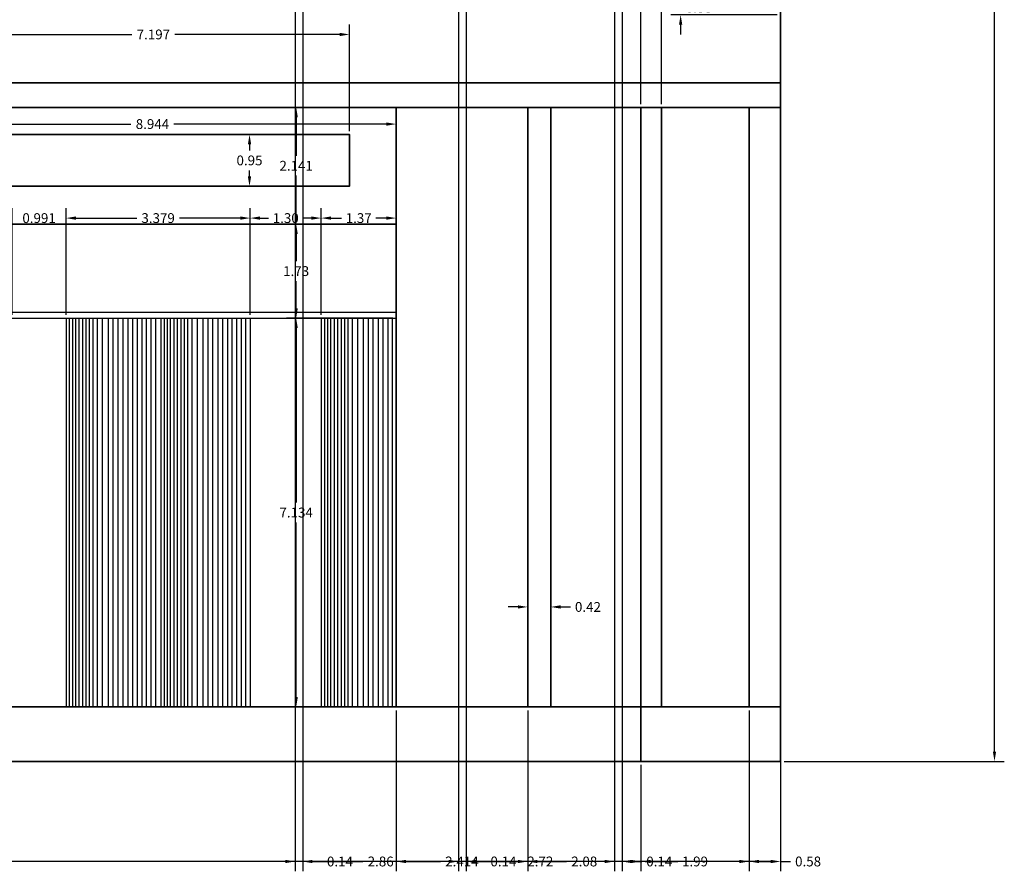
# Model space of a CAD drawing. Units: millimetres. Extents: x 2473 to 2512.3, y 2191.3 to 2230.4.
# Tile 6 of 8: x 2493.7 to 2511.7, y 2191.3 to 2207. Entities that reach past the tile are written whole.
import ezdxf

# ---------------------------------------------------------------- set-up
doc = ezdxf.new("R2010")
doc.units = ezdxf.units.MM
for name, color, linetype, lineweight in [('A-ANNO-DIMS', 2, 'Continuous', 18), ('A-DOOR', 4, 'Continuous', 25), ('A-ELEV', 7, 'Continuous', 35)]:
    doc.layers.add(name, color=color, linetype=linetype, lineweight=lineweight)
doc.styles.get("Standard").update_dxf_attribs({"font": 'arial.ttf'})
doc.dimstyles.get("Standard").update_dxf_attribs({"dimtxt": 0.18, "dimasz": 0.18, "dimexe": 0.18, "dimexo": 0.0625, "dimgap": 0.09, "dimtad": 0, "dimtih": 1, "dimtoh": 1, "dimdec": 4, "dimzin": 0, "dimdsep": 46, "dimtxsty": 'Standard', "dimcen": 0.09, "dimadec": 0, "dimazin": 0, "dimtfac": 1, "dimtdec": 4, "dimtofl": 0, "dimtmove": 0, "dimatfit": 3, "dimfxl": 1, "dimtolj": 1, "dimtzin": 0, "dimarcsym": 0})

# ---------------------------------------------------------------- blocks, each defined once
blk = doc.blocks.new('*D7')
at = {"layer": 'A-ANNO-DIMS', "color": 0, "lineweight": -2, "transparency": 16777216}
for p, q in [((2475.623, 2193.292), (2475.623, 2191.34)), ((2507.623, 2193.292), (2507.623, 2191.34)), ((2475.803, 2191.52), (2491.405, 2191.52)), ((2507.443, 2191.52), (2491.841, 2191.52))]:
    blk.add_line(p, q, dxfattribs=at)
at = {"layer": 'A-ANNO-DIMS', "color": 0, "transparency": 16777216}
for points in [[(2475.803, 2191.55), (2475.803, 2191.49), (2475.623, 2191.52)], [(2507.443, 2191.55), (2507.443, 2191.49), (2507.623, 2191.52)]]:
    blk.add_solid(points, dxfattribs=at)
at = {"layer": 'Defpoints', "color": 0, "transparency": 16777216}
for p in [(2475.623, 2193.355), (2507.623, 2193.355), (2507.623, 2191.52)]:
    blk.add_point(p, dxfattribs=at)
at = {"layer": 'A-ANNO-DIMS', "color": 0, "transparency": 16777216, "insert": (2491.623, 2191.52), "char_height": 0.18, "attachment_point": 5}
blk.add_mtext('\\A1;32', dxfattribs=at)
blk = doc.blocks.new('*D9')
at = {"layer": 'A-ANNO-DIMS', "color": 0, "lineweight": -2, "transparency": 16777216}
for p, q in [((2509.775, 2228.355), (2511.728, 2228.355)), ((2511.548, 2228.175), (2511.548, 2211.037)), ((2511.548, 2193.535), (2511.548, 2210.673)), ((2507.685, 2193.355), (2511.728, 2193.355))]:
    blk.add_line(p, q, dxfattribs=at)
at = {"layer": 'A-ANNO-DIMS', "color": 0, "transparency": 16777216}
for points in [[(2511.518, 2228.175), (2511.578, 2228.175), (2511.548, 2228.355)], [(2511.518, 2193.535), (2511.578, 2193.535), (2511.548, 2193.355)]]:
    blk.add_solid(points, dxfattribs=at)
at = {"layer": 'Defpoints', "color": 0, "transparency": 16777216}
for p in [(2509.713, 2228.355), (2511.548, 2228.355), (2507.623, 2193.355)]:
    blk.add_point(p, dxfattribs=at)
at = {"layer": 'A-ANNO-DIMS', "color": 0, "transparency": 16777216, "insert": (2511.548, 2210.855), "char_height": 0.18, "attachment_point": 5}
blk.add_mtext('\\A1;35', dxfattribs=at)
blk = doc.blocks.new('*D16')
at = {"layer": 'A-ANNO-DIMS', "color": 0, "lineweight": -2, "transparency": 16777216}
for p, q in [((2491.623, 2203.276), (2491.623, 2205.229)), ((2500.567, 2203.276), (2500.567, 2205.229)), ((2491.803, 2205.049), (2495.701, 2205.049)), ((2500.387, 2205.049), (2496.488, 2205.049))]:
    blk.add_line(p, q, dxfattribs=at)
at = {"layer": 'A-ANNO-DIMS', "color": 0, "transparency": 16777216}
for points in [[(2491.803, 2205.079), (2491.803, 2205.019), (2491.623, 2205.049)], [(2500.387, 2205.079), (2500.387, 2205.019), (2500.567, 2205.049)]]:
    blk.add_solid(points, dxfattribs=at)
at = {"layer": 'Defpoints', "color": 0, "transparency": 16777216}
for p in [(2500.567, 2205.049), (2491.623, 2203.214), (2500.567, 2203.214)]:
    blk.add_point(p, dxfattribs=at)
at = {"layer": 'A-ANNO-DIMS', "color": 0, "transparency": 16777216, "insert": (2496.095, 2205.049), "char_height": 0.18, "attachment_point": 5}
blk.add_mtext('\\A1;8.944', dxfattribs=at)
blk = doc.blocks.new('*D26')
at = {"layer": 'A-ANNO-DIMS', "color": 0, "lineweight": -2, "transparency": 16777216}
for p, q in [((2500.567, 2194.292), (2500.567, 2191.34)), ((2502.981, 2194.292), (2502.981, 2191.34)), ((2500.747, 2191.52), (2501.379, 2191.52)), ((2502.801, 2191.52), (2502.169, 2191.52))]:
    blk.add_line(p, q, dxfattribs=at)
at = {"layer": 'A-ANNO-DIMS', "color": 0, "transparency": 16777216}
for points in [[(2500.747, 2191.55), (2500.747, 2191.49), (2500.567, 2191.52)], [(2502.801, 2191.55), (2502.801, 2191.49), (2502.981, 2191.52)]]:
    blk.add_solid(points, dxfattribs=at)
at = {"layer": 'Defpoints', "color": 0, "transparency": 16777216}
for p in [(2500.567, 2194.355), (2502.981, 2194.355), (2502.981, 2191.52)]:
    blk.add_point(p, dxfattribs=at)
at = {"layer": 'A-ANNO-DIMS', "color": 0, "transparency": 16777216, "insert": (2501.774, 2191.52), "char_height": 0.18, "attachment_point": 5}
blk.add_mtext('\\A1;2.414', dxfattribs=at)
blk = doc.blocks.new('*D27')
at = {"layer": 'A-ANNO-DIMS', "color": 0, "lineweight": -2, "transparency": 16777216}
for p, q in [((2502.981, 2194.292), (2502.981, 2191.34)), ((2505.056, 2193.292), (2505.056, 2191.34)), ((2503.161, 2191.52), (2503.693, 2191.52)), ((2504.876, 2191.52), (2504.344, 2191.52))]:
    blk.add_line(p, q, dxfattribs=at)
at = {"layer": 'A-ANNO-DIMS', "color": 0, "transparency": 16777216}
for points in [[(2503.161, 2191.55), (2503.161, 2191.49), (2502.981, 2191.52)], [(2504.876, 2191.55), (2504.876, 2191.49), (2505.056, 2191.52)]]:
    blk.add_solid(points, dxfattribs=at)
at = {"layer": 'Defpoints', "color": 0, "transparency": 16777216}
for p in [(2502.981, 2194.355), (2505.056, 2193.355), (2505.056, 2191.52)]:
    blk.add_point(p, dxfattribs=at)
at = {"layer": 'A-ANNO-DIMS', "color": 0, "transparency": 16777216, "insert": (2504.019, 2191.52), "char_height": 0.18, "attachment_point": 5}
blk.add_mtext('\\A1;2.08', dxfattribs=at)
blk = doc.blocks.new('*D28')
at = {"layer": 'A-ANNO-DIMS', "color": 0, "lineweight": -2, "transparency": 16777216}
for p, q in [((2507.047, 2194.292), (2507.047, 2191.34)), ((2505.056, 2193.292), (2505.056, 2191.34)), ((2505.236, 2191.52), (2505.736, 2191.52)), ((2506.867, 2191.52), (2506.367, 2191.52))]:
    blk.add_line(p, q, dxfattribs=at)
at = {"layer": 'A-ANNO-DIMS', "color": 0, "transparency": 16777216}
for points in [[(2505.236, 2191.55), (2505.236, 2191.49), (2505.056, 2191.52)], [(2506.867, 2191.55), (2506.867, 2191.49), (2507.047, 2191.52)]]:
    blk.add_solid(points, dxfattribs=at)
at = {"layer": 'Defpoints', "color": 0, "transparency": 16777216}
for p in [(2507.047, 2194.355), (2505.056, 2193.355), (2507.047, 2191.52)]:
    blk.add_point(p, dxfattribs=at)
at = {"layer": 'A-ANNO-DIMS', "color": 0, "transparency": 16777216, "insert": (2506.052, 2191.52), "char_height": 0.18, "attachment_point": 5}
blk.add_mtext('\\A1;1.99', dxfattribs=at)
blk = doc.blocks.new('*D29')
at = {"layer": 'A-ANNO-DIMS', "color": 0, "lineweight": -2, "transparency": 16777216}
for p, q in [((2507.047, 2194.292), (2507.047, 2191.34)), ((2507.623, 2194.292), (2507.623, 2191.34)), ((2507.227, 2191.52), (2507.443, 2191.52)), ((2507.623, 2191.52), (2507.803, 2191.52))]:
    blk.add_line(p, q, dxfattribs=at)
at = {"layer": 'A-ANNO-DIMS', "color": 0, "transparency": 16777216}
for points in [[(2507.227, 2191.55), (2507.227, 2191.49), (2507.047, 2191.52)], [(2507.443, 2191.55), (2507.443, 2191.49), (2507.623, 2191.52)]]:
    blk.add_solid(points, dxfattribs=at)
at = {"layer": 'Defpoints', "color": 0, "transparency": 16777216}
for p in [(2507.047, 2194.355), (2507.623, 2194.355), (2507.623, 2191.52)]:
    blk.add_point(p, dxfattribs=at)
at = {"layer": 'A-ANNO-DIMS', "color": 0, "transparency": 16777216, "insert": (2508.127, 2191.52), "char_height": 0.18, "attachment_point": 5}
blk.add_mtext('\\A1;0.58', dxfattribs=at)
blk = doc.blocks.new('*D30')
at = {"layer": 'A-ANNO-DIMS', "color": 0, "lineweight": -2, "transparency": 16777216}
for p, q in [((2502.981, 2194.417), (2502.981, 2196.37)), ((2503.405, 2194.417), (2503.405, 2196.37)), ((2502.801, 2196.19), (2502.621, 2196.19)), ((2503.585, 2196.19), (2503.765, 2196.19))]:
    blk.add_line(p, q, dxfattribs=at)
at = {"layer": 'A-ANNO-DIMS', "color": 0, "transparency": 16777216}
for points in [[(2502.801, 2196.22), (2502.801, 2196.16), (2502.981, 2196.19)], [(2503.585, 2196.22), (2503.585, 2196.16), (2503.405, 2196.19)]]:
    blk.add_solid(points, dxfattribs=at)
at = {"layer": 'Defpoints', "color": 0, "transparency": 16777216}
for p in [(2503.405, 2196.19), (2502.981, 2194.355), (2503.405, 2194.355)]:
    blk.add_point(p, dxfattribs=at)
at = {"layer": 'A-ANNO-DIMS', "color": 0, "transparency": 16777216, "insert": (2504.087, 2196.19), "char_height": 0.18, "attachment_point": 5}
blk.add_mtext('\\A1;0.42', dxfattribs=at)
blk = doc.blocks.new('*D31')
at = {"layer": 'A-ANNO-DIMS', "color": 0, "lineweight": -2, "transparency": 16777216}
for p, q in [((2505.056, 2205.417), (2505.056, 2207.37)), ((2505.438, 2205.417), (2505.438, 2207.37)), ((2504.876, 2207.19), (2504.696, 2207.19)), ((2505.618, 2207.19), (2505.798, 2207.19))]:
    blk.add_line(p, q, dxfattribs=at)
at = {"layer": 'A-ANNO-DIMS', "color": 0, "transparency": 16777216}
for points in [[(2504.876, 2207.22), (2504.876, 2207.16), (2505.056, 2207.19)], [(2505.618, 2207.22), (2505.618, 2207.16), (2505.438, 2207.19)]]:
    blk.add_solid(points, dxfattribs=at)
at = {"layer": 'Defpoints', "color": 0, "transparency": 16777216}
for p in [(2505.438, 2207.19), (2505.056, 2205.355), (2505.438, 2205.355)]:
    blk.add_point(p, dxfattribs=at)
at = {"layer": 'A-ANNO-DIMS', "color": 0, "transparency": 16777216, "insert": (2506.122, 2207.19), "char_height": 0.18, "attachment_point": 5}
blk.add_mtext('\\A1;0.38', dxfattribs=at)
blk = doc.blocks.new('*D33')
at = {"layer": 'A-ANNO-DIMS', "color": 0, "lineweight": -2, "transparency": 16777216}
for p, q in [((2493.518828, 2201.551016), (2493.518828, 2203.503516)), ((2494.509822, 2201.551016), (2494.509822, 2203.503516)), ((2493.338828, 2203.323516), (2493.158828, 2203.323516)), ((2494.689822, 2203.323516), (2494.869822, 2203.323516))]:
    blk.add_line(p, q, dxfattribs=at)
at = {"layer": 'A-ANNO-DIMS', "color": 0, "transparency": 16777216}
for points in [[(2493.338828, 2203.353516), (2493.338828, 2203.293516), (2493.518828, 2203.323516)], [(2494.689822, 2203.353516), (2494.689822, 2203.293516), (2494.509822, 2203.323516)]]:
    blk.add_solid(points, dxfattribs=at)
at = {"layer": 'Defpoints', "color": 0, "transparency": 16777216}
for p in [(2494.509822, 2203.323516), (2493.518828, 2201.488516), (2494.509822, 2201.488516)]:
    blk.add_point(p, dxfattribs=at)
at = {"layer": 'A-ANNO-DIMS', "color": 0, "transparency": 16777216, "insert": (2494.014325, 2203.323516), "char_height": 0.18, "attachment_point": 5}
blk.add_mtext('\\A1;0.991', dxfattribs=at)
blk = doc.blocks.new('*D34')
at = {"layer": 'A-ANNO-DIMS', "color": 0, "lineweight": -2, "transparency": 16777216}
for p, q in [((2494.51, 2201.551), (2494.51, 2203.504)), ((2497.889, 2201.551), (2497.889, 2203.504)), ((2494.69, 2203.324), (2495.806, 2203.324)), ((2497.709, 2203.324), (2496.593, 2203.324))]:
    blk.add_line(p, q, dxfattribs=at)
at = {"layer": 'A-ANNO-DIMS', "color": 0, "transparency": 16777216}
for points in [[(2494.69, 2203.354), (2494.69, 2203.294), (2494.51, 2203.324)], [(2497.709, 2203.354), (2497.709, 2203.294), (2497.889, 2203.324)]]:
    blk.add_solid(points, dxfattribs=at)
at = {"layer": 'Defpoints', "color": 0, "transparency": 16777216}
for p in [(2497.889, 2203.324), (2494.51, 2201.489), (2497.889, 2201.489)]:
    blk.add_point(p, dxfattribs=at)
at = {"layer": 'A-ANNO-DIMS', "color": 0, "transparency": 16777216, "insert": (2496.199, 2203.324), "char_height": 0.18, "attachment_point": 5}
blk.add_mtext('\\A1;3.379', dxfattribs=at)
blk = doc.blocks.new('*D35')
at = {"layer": 'A-ANNO-DIMS', "color": 0, "lineweight": -2, "transparency": 16777216}
for p, q in [((2497.889, 2201.551), (2497.889, 2203.504)), ((2499.192, 2201.551), (2499.192, 2203.504)), ((2498.069, 2203.324), (2498.226, 2203.324)), ((2499.012, 2203.324), (2498.856, 2203.324))]:
    blk.add_line(p, q, dxfattribs=at)
at = {"layer": 'A-ANNO-DIMS', "color": 0, "transparency": 16777216}
for points in [[(2498.069, 2203.354), (2498.069, 2203.294), (2497.889, 2203.324)], [(2499.012, 2203.354), (2499.012, 2203.294), (2499.192, 2203.324)]]:
    blk.add_solid(points, dxfattribs=at)
at = {"layer": 'Defpoints', "color": 0, "transparency": 16777216}
for p in [(2499.192, 2203.324), (2497.889, 2201.489), (2499.192, 2201.489)]:
    blk.add_point(p, dxfattribs=at)
at = {"layer": 'A-ANNO-DIMS', "color": 0, "transparency": 16777216, "insert": (2498.541, 2203.324), "char_height": 0.18, "attachment_point": 5}
blk.add_mtext('\\A1;1.30', dxfattribs=at)
blk = doc.blocks.new('*D36')
at = {"layer": 'A-ANNO-DIMS', "color": 0, "lineweight": -2, "transparency": 16777216}
for p, q in [((2499.192, 2201.551), (2499.192, 2203.504)), ((2500.567, 2201.551), (2500.567, 2203.504)), ((2499.372, 2203.324), (2499.564, 2203.324)), ((2500.387, 2203.324), (2500.195, 2203.324))]:
    blk.add_line(p, q, dxfattribs=at)
at = {"layer": 'A-ANNO-DIMS', "color": 0, "transparency": 16777216}
for points in [[(2499.372, 2203.354), (2499.372, 2203.294), (2499.192, 2203.324)], [(2500.387, 2203.354), (2500.387, 2203.294), (2500.567, 2203.324)]]:
    blk.add_solid(points, dxfattribs=at)
at = {"layer": 'Defpoints', "color": 0, "transparency": 16777216}
for p in [(2500.567, 2203.324), (2499.192, 2201.489), (2500.567, 2201.489)]:
    blk.add_point(p, dxfattribs=at)
at = {"layer": 'A-ANNO-DIMS', "color": 0, "transparency": 16777216, "insert": (2499.88, 2203.324), "char_height": 0.18, "attachment_point": 5}
blk.add_mtext('\\A1;1.37', dxfattribs=at)
blk = doc.blocks.new('*D39')
at = {"layer": 'A-ANNO-DIMS', "color": 0, "lineweight": -2, "transparency": 16777216}
for p, q in [((2500.504, 2201.489), (2498.552, 2201.489)), ((2498.732, 2201.309), (2498.732, 2198.104)), ((2498.732, 2194.535), (2498.732, 2197.74)), ((2500.504, 2194.355), (2498.552, 2194.355))]:
    blk.add_line(p, q, dxfattribs=at)
at = {"layer": 'A-ANNO-DIMS', "color": 0, "transparency": 16777216}
for points in [[(2498.702, 2201.309), (2498.762, 2201.309), (2498.732, 2201.489)], [(2498.702, 2194.535), (2498.762, 2194.535), (2498.732, 2194.355)]]:
    blk.add_solid(points, dxfattribs=at)
at = {"layer": 'Defpoints', "color": 0, "transparency": 16777216}
for p in [(2498.732, 2201.489), (2500.567, 2201.489), (2500.567, 2194.355)]:
    blk.add_point(p, dxfattribs=at)
at = {"layer": 'A-ANNO-DIMS', "color": 0, "transparency": 16777216, "insert": (2498.732, 2197.922), "char_height": 0.18, "attachment_point": 5}
blk.add_mtext('\\A1;7.134', dxfattribs=at)
blk = doc.blocks.new('*D40')
at = {"layer": 'A-ANNO-DIMS', "color": 0, "lineweight": -2, "transparency": 16777216}
for p, q in [((2500.504, 2203.214), (2498.552, 2203.214)), ((2498.732, 2203.034), (2498.732, 2202.533)), ((2498.732, 2201.669), (2498.732, 2202.169)), ((2500.504, 2201.489), (2498.552, 2201.489))]:
    blk.add_line(p, q, dxfattribs=at)
at = {"layer": 'A-ANNO-DIMS', "color": 0, "transparency": 16777216}
for points in [[(2498.702, 2203.034), (2498.762, 2203.034), (2498.732, 2203.214)], [(2498.702, 2201.669), (2498.762, 2201.669), (2498.732, 2201.489)]]:
    blk.add_solid(points, dxfattribs=at)
at = {"layer": 'Defpoints', "color": 0, "transparency": 16777216}
for p in [(2498.732, 2203.214), (2500.567, 2203.214), (2500.567, 2201.489)]:
    blk.add_point(p, dxfattribs=at)
at = {"layer": 'A-ANNO-DIMS', "color": 0, "transparency": 16777216, "insert": (2498.732, 2202.351), "char_height": 0.18, "attachment_point": 5}
blk.add_mtext('\\A1;1.73', dxfattribs=at)
blk = doc.blocks.new('*D41')
at = {"layer": 'A-ANNO-DIMS', "color": 0, "lineweight": -2, "transparency": 16777216}
for p, q in [((2500.504, 2205.355), (2498.552, 2205.355)), ((2498.732, 2205.175), (2498.732, 2204.465)), ((2498.732, 2203.394), (2498.732, 2204.104)), ((2500.504, 2203.214), (2498.552, 2203.214))]:
    blk.add_line(p, q, dxfattribs=at)
at = {"layer": 'A-ANNO-DIMS', "color": 0, "transparency": 16777216}
for points in [[(2498.702, 2205.175), (2498.762, 2205.175), (2498.732, 2205.355)], [(2498.702, 2203.394), (2498.762, 2203.394), (2498.732, 2203.214)]]:
    blk.add_solid(points, dxfattribs=at)
at = {"layer": 'Defpoints', "color": 0, "transparency": 16777216}
for p in [(2498.732, 2205.355), (2500.567, 2205.355), (2500.567, 2203.214)]:
    blk.add_point(p, dxfattribs=at)
at = {"layer": 'A-ANNO-DIMS', "color": 0, "transparency": 16777216, "insert": (2498.732, 2204.284), "char_height": 0.18, "attachment_point": 5}
blk.add_mtext('\\A1;2.141', dxfattribs=at)
blk = doc.blocks.new('*D42')
at = {"layer": 'A-ANNO-DIMS', "color": 0, "lineweight": -2, "transparency": 16777216}
for p, q in [((2499.648, 2204.858), (2497.696, 2204.858)), ((2497.876, 2204.678), (2497.876, 2204.564)), ((2497.876, 2204.087), (2497.876, 2204.2)), ((2499.648, 2203.907), (2497.696, 2203.907))]:
    blk.add_line(p, q, dxfattribs=at)
at = {"layer": 'A-ANNO-DIMS', "color": 0, "transparency": 16777216}
for points in [[(2497.846, 2204.678), (2497.906, 2204.678), (2497.876, 2204.858)], [(2497.846, 2204.087), (2497.906, 2204.087), (2497.876, 2203.907)]]:
    blk.add_solid(points, dxfattribs=at)
at = {"layer": 'Defpoints', "color": 0, "transparency": 16777216}
for p in [(2497.876, 2204.858), (2499.711, 2204.858), (2499.711, 2203.907)]:
    blk.add_point(p, dxfattribs=at)
at = {"layer": 'A-ANNO-DIMS', "color": 0, "transparency": 16777216, "insert": (2497.876, 2204.382), "char_height": 0.18, "attachment_point": 5}
blk.add_mtext('\\A1;0.95', dxfattribs=at)
blk = doc.blocks.new('*D44')
at = {"layer": 'A-ANNO-DIMS', "color": 0, "lineweight": -2, "transparency": 16777216}
for p, q in [((2492.513, 2204.92), (2492.513, 2206.873)), ((2499.711, 2204.92), (2499.711, 2206.873)), ((2492.693, 2206.693), (2495.719, 2206.693)), ((2499.531, 2206.693), (2496.505, 2206.693))]:
    blk.add_line(p, q, dxfattribs=at)
at = {"layer": 'A-ANNO-DIMS', "color": 0, "transparency": 16777216}
for points in [[(2492.693, 2206.723), (2492.693, 2206.663), (2492.513, 2206.693)], [(2499.531, 2206.723), (2499.531, 2206.663), (2499.711, 2206.693)]]:
    blk.add_solid(points, dxfattribs=at)
at = {"layer": 'Defpoints', "color": 0, "transparency": 16777216}
for p in [(2499.711, 2206.693), (2492.513, 2204.858), (2499.711, 2204.858)]:
    blk.add_point(p, dxfattribs=at)
at = {"layer": 'A-ANNO-DIMS', "color": 0, "transparency": 16777216, "insert": (2496.112, 2206.693), "char_height": 0.18, "attachment_point": 5}
blk.add_mtext('\\A1;7.197', dxfattribs=at)
blk = doc.blocks.new('*D61')
at = {"layer": 'A-ANNO-DIMS', "color": 0, "lineweight": -2, "transparency": 16777216}
for p, q in [((2505.788, 2207.687), (2505.788, 2207.867)), ((2507.56, 2207.507), (2505.608, 2207.507)), ((2507.56, 2207.055), (2505.608, 2207.055)), ((2505.788, 2206.875), (2505.788, 2206.695))]:
    blk.add_line(p, q, dxfattribs=at)
at = {"layer": 'A-ANNO-DIMS', "color": 0, "transparency": 16777216}
for points in [[(2505.758, 2207.687), (2505.818, 2207.687), (2505.788, 2207.507)], [(2505.758, 2206.875), (2505.818, 2206.875), (2505.788, 2207.055)]]:
    blk.add_solid(points, dxfattribs=at)
at = {"layer": 'Defpoints', "color": 0, "transparency": 16777216}
for p in [(2505.788, 2207.507), (2507.623, 2207.507), (2507.623, 2207.055)]:
    blk.add_point(p, dxfattribs=at)
at = {"layer": 'A-ANNO-DIMS', "color": 0, "transparency": 16777216, "insert": (2505.788, 2207.281), "char_height": 0.18, "attachment_point": 5}
blk.add_mtext('\\A1;0.452', dxfattribs=at)
blk = doc.blocks.new('*D115')
at = {"layer": 'A-ANNO-DIMS', "color": 0, "lineweight": -2, "transparency": 16777216}
for p, q in [((2498.713, 2222.992), (2498.713, 2191.34)), ((2498.852, 2222.992), (2498.852, 2191.34)), ((2498.533, 2191.52), (2498.353, 2191.52)), ((2499.032, 2191.52), (2499.212, 2191.52))]:
    blk.add_line(p, q, dxfattribs=at)
at = {"layer": 'A-ANNO-DIMS', "color": 0, "transparency": 16777216}
for points in [[(2498.533, 2191.55), (2498.533, 2191.49), (2498.713, 2191.52)], [(2499.032, 2191.55), (2499.032, 2191.49), (2498.852, 2191.52)]]:
    blk.add_solid(points, dxfattribs=at)
at = {"layer": 'Defpoints', "color": 0, "transparency": 16777216}
for p in [(2498.713, 2223.055), (2498.852, 2223.055), (2498.852, 2191.52)]:
    blk.add_point(p, dxfattribs=at)
at = {"layer": 'A-ANNO-DIMS', "color": 0, "transparency": 16777216, "insert": (2499.536, 2191.52), "char_height": 0.18, "attachment_point": 5}
blk.add_mtext('\\A1;0.14', dxfattribs=at)
blk = doc.blocks.new('*D116')
at = {"layer": 'A-ANNO-DIMS', "color": 0, "lineweight": -2, "transparency": 16777216}
for p, q in [((2498.852, 2222.992), (2498.852, 2191.34)), ((2501.713, 2222.992), (2501.713, 2191.34)), ((2499.032, 2191.52), (2499.957, 2191.52)), ((2501.533, 2191.52), (2500.608, 2191.52))]:
    blk.add_line(p, q, dxfattribs=at)
at = {"layer": 'A-ANNO-DIMS', "color": 0, "transparency": 16777216}
for points in [[(2499.032, 2191.55), (2499.032, 2191.49), (2498.852, 2191.52)], [(2501.533, 2191.55), (2501.533, 2191.49), (2501.713, 2191.52)]]:
    blk.add_solid(points, dxfattribs=at)
at = {"layer": 'Defpoints', "color": 0, "transparency": 16777216}
for p in [(2498.852, 2223.055), (2501.713, 2223.055), (2501.713, 2191.52)]:
    blk.add_point(p, dxfattribs=at)
at = {"layer": 'A-ANNO-DIMS', "color": 0, "transparency": 16777216, "insert": (2500.283, 2191.52), "char_height": 0.18, "attachment_point": 5}
blk.add_mtext('\\A1;2.86', dxfattribs=at)
blk = doc.blocks.new('*D117')
at = {"layer": 'A-ANNO-DIMS', "color": 0, "lineweight": -2, "transparency": 16777216}
for p, q in [((2501.713, 2222.992), (2501.713, 2191.34)), ((2501.853, 2222.992), (2501.853, 2191.34)), ((2501.533, 2191.52), (2501.353, 2191.52)), ((2502.033, 2191.52), (2502.213, 2191.52))]:
    blk.add_line(p, q, dxfattribs=at)
at = {"layer": 'A-ANNO-DIMS', "color": 0, "transparency": 16777216}
for points in [[(2501.533, 2191.55), (2501.533, 2191.49), (2501.713, 2191.52)], [(2502.033, 2191.55), (2502.033, 2191.49), (2501.853, 2191.52)]]:
    blk.add_solid(points, dxfattribs=at)
at = {"layer": 'Defpoints', "color": 0, "transparency": 16777216}
for p in [(2501.713, 2223.055), (2501.853, 2223.055), (2501.853, 2191.52)]:
    blk.add_point(p, dxfattribs=at)
at = {"layer": 'A-ANNO-DIMS', "color": 0, "transparency": 16777216, "insert": (2502.536, 2191.52), "char_height": 0.18, "attachment_point": 5}
blk.add_mtext('\\A1;0.14', dxfattribs=at)
blk = doc.blocks.new('*D118')
at = {"layer": 'A-ANNO-DIMS', "color": 0, "lineweight": -2, "transparency": 16777216}
for p, q in [((2501.853, 2222.992), (2501.853, 2191.34)), ((2504.573, 2222.992), (2504.573, 2191.34)), ((2502.033, 2191.52), (2502.888, 2191.52)), ((2504.393, 2191.52), (2503.537, 2191.52))]:
    blk.add_line(p, q, dxfattribs=at)
at = {"layer": 'A-ANNO-DIMS', "color": 0, "transparency": 16777216}
for points in [[(2502.033, 2191.55), (2502.033, 2191.49), (2501.853, 2191.52)], [(2504.393, 2191.55), (2504.393, 2191.49), (2504.573, 2191.52)]]:
    blk.add_solid(points, dxfattribs=at)
at = {"layer": 'Defpoints', "color": 0, "transparency": 16777216}
for p in [(2501.853, 2223.055), (2504.573, 2223.055), (2504.573, 2191.52)]:
    blk.add_point(p, dxfattribs=at)
at = {"layer": 'A-ANNO-DIMS', "color": 0, "transparency": 16777216, "insert": (2503.213, 2191.52), "char_height": 0.18, "attachment_point": 5}
blk.add_mtext('\\A1;2.72', dxfattribs=at)
blk = doc.blocks.new('*D119')
at = {"layer": 'A-ANNO-DIMS', "color": 0, "lineweight": -2, "transparency": 16777216}
for p, q in [((2504.573, 2222.992), (2504.573, 2191.34)), ((2504.713, 2222.992), (2504.713, 2191.34)), ((2504.393, 2191.52), (2504.213, 2191.52)), ((2504.893, 2191.52), (2505.073, 2191.52))]:
    blk.add_line(p, q, dxfattribs=at)
at = {"layer": 'A-ANNO-DIMS', "color": 0, "transparency": 16777216}
for points in [[(2504.393, 2191.55), (2504.393, 2191.49), (2504.573, 2191.52)], [(2504.893, 2191.55), (2504.893, 2191.49), (2504.713, 2191.52)]]:
    blk.add_solid(points, dxfattribs=at)
at = {"layer": 'Defpoints', "color": 0, "transparency": 16777216}
for p in [(2504.573, 2223.055), (2504.713, 2223.055), (2504.713, 2191.52)]:
    blk.add_point(p, dxfattribs=at)
at = {"layer": 'A-ANNO-DIMS', "color": 0, "transparency": 16777216, "insert": (2505.396, 2191.52), "char_height": 0.18, "attachment_point": 5}
blk.add_mtext('\\A1;0.14', dxfattribs=at)

msp = doc.modelspace()

# ---------------------------------------------------------------- linework, layer by layer
at = {"layer": 'A-DOOR'}
for p, q in [((2491.6229, 2201.5952), (2500.5668, 2201.5952)), ((2491.6229, 2201.4885), (2500.5668, 2201.4885)), ((2494.5098, 2201.4885), (2494.5098, 2194.3549)), ((2494.5685, 2201.4885), (2494.5685, 2194.3549)), ((2494.6272, 2201.4885), (2494.6272, 2194.3549)), ((2494.6807, 2201.4885), (2494.6807, 2194.3549)), ((2494.7445, 2201.4885), (2494.7445, 2194.3549)), ((2494.8084, 2201.4885), (2494.8084, 2194.3549)), ((2494.874, 2201.4885), (2494.874, 2194.3549)), ((2494.9361, 2201.4885), (2494.9361, 2194.3549)), ((2494.9994, 2201.4885), (2494.9994, 2194.3549)), ((2495.0785, 2201.4885), (2495.0785, 2194.3549)), ((2495.174, 2201.4885), (2495.174, 2194.3549)), ((2495.2804, 2201.4885), (2495.2804, 2194.3549)), ((2495.3704, 2201.4885), (2495.3704, 2194.3549)), ((2495.4577, 2201.4885), (2495.4577, 2194.3549)), ((2495.5531, 2201.4885), (2495.5531, 2194.3549)), ((2495.6404, 2201.4885), (2495.6404, 2194.3549)), ((2495.7304, 2201.4885), (2495.7304, 2194.3549)), ((2495.8123, 2201.4885), (2495.8123, 2194.3549)), ((2495.8995, 2201.4885), (2495.8995, 2194.3549)), ((2495.9814, 2201.4885), (2495.9814, 2194.3549)), ((2496.0632, 2201.4885), (2496.0632, 2194.3549)), ((2496.1493, 2201.4885), (2496.1493, 2194.3549)), ((2496.2496, 2201.4885), (2496.2496, 2194.3549)), ((2496.3083, 2201.4885), (2496.3083, 2194.3549)), ((2496.3669, 2201.4885), (2496.3669, 2194.3549)), ((2496.4204, 2201.4885), (2496.4204, 2194.3549)), ((2496.4843, 2201.4885), (2496.4843, 2194.3549)), ((2496.5481, 2201.4885), (2496.5481, 2194.3549)), ((2496.6137, 2201.4885), (2496.6137, 2194.3549)), ((2496.6758, 2201.4885), (2496.6758, 2194.3549)), ((2496.7392, 2201.4885), (2496.7392, 2194.3549)), ((2496.8183, 2201.4885), (2496.8183, 2194.3549)), ((2496.9137, 2201.4885), (2496.9137, 2194.3549)), ((2497.0201, 2201.4885), (2497.0201, 2194.3549)), ((2497.1101, 2201.4885), (2497.1101, 2194.3549)), ((2497.1974, 2201.4885), (2497.1974, 2194.3549)), ((2497.2929, 2201.4885), (2497.2929, 2194.3549)), ((2497.3802, 2201.4885), (2497.3802, 2194.3549)), ((2497.4702, 2201.4885), (2497.4702, 2194.3549)), ((2497.552, 2201.4885), (2497.552, 2194.3549)), ((2497.6393, 2201.4885), (2497.6393, 2194.3549)), ((2497.7211, 2201.4885), (2497.7211, 2194.3549)), ((2497.8029, 2201.4885), (2497.8029, 2194.3549)), ((2497.889, 2201.4885), (2497.889, 2194.3549)), ((2499.1923, 2201.4885), (2499.1923, 2194.3549)), ((2499.251, 2201.4885), (2499.251, 2194.3549)), ((2499.3097, 2201.4885), (2499.3097, 2194.3549)), ((2499.3632, 2201.4885), (2499.3632, 2194.3549)), ((2499.4271, 2201.4885), (2499.4271, 2194.3549)), ((2499.4909, 2201.4885), (2499.4909, 2194.3549)), ((2499.5565, 2201.4885), (2499.5565, 2194.3549)), ((2499.6186, 2201.4885), (2499.6186, 2194.3549)), ((2499.682, 2201.4885), (2499.682, 2194.3549)), ((2499.7611, 2201.4885), (2499.7611, 2194.3549)), ((2499.8565, 2201.4885), (2499.8565, 2194.3549)), ((2499.9629, 2201.4885), (2499.9629, 2194.3549)), ((2500.0529, 2201.4885), (2500.0529, 2194.3549)), ((2500.1402, 2201.4885), (2500.1402, 2194.3549)), ((2500.2357, 2201.4885), (2500.2357, 2194.3549)), ((2500.3229, 2201.4885), (2500.3229, 2194.3549)), ((2500.4129, 2201.4885), (2500.4129, 2194.3549)), ((2500.4948, 2201.4885), (2500.4948, 2194.3549))]:
    msp.add_line(p, q, dxfattribs=at)
at = {"layer": 'A-ELEV'}
for p, q in [((2507.6229, 2219.0549), (2507.6229, 2193.3549)), ((2507.6229, 2205.8077), (2475.6229, 2205.8077)), ((2507.6229, 2205.3549), (2475.6229, 2205.3549)), ((2500.5668, 2205.3549), (2500.5668, 2194.3549)), ((2502.9811, 2205.3549), (2502.9811, 2194.3549)), ((2503.4046, 2194.3549), (2503.4046, 2205.3549)), ((2505.0565, 2193.3549), (2505.0565, 2205.3549)), ((2505.4377, 2194.3549), (2505.4377, 2205.3549)), ((2507.0472, 2194.3549), (2507.0472, 2205.3549)), ((2491.6229, 2203.2139), (2500.5668, 2203.2139)), ((2507.6229, 2194.3549), (2491.6229, 2194.3549)), ((2507.6229, 2193.3549), (2475.6229, 2193.3549))]:
    msp.add_line(p, q, dxfattribs=at)
msp.add_lwpolyline([(2492.5133, 2204.8576), (2499.7107, 2204.8576), (2499.7107, 2203.907), (2492.5133, 2203.907)], close=True, dxfattribs=at)

# ---------------------------------------------------------------- dimensions: what is measured, and where the dimension line sits
at = {"layer": 'A-ANNO-DIMS'}
for base, p1, p2, override, picture, middle in [((2511.5479, 2228.3549), (2507.6229, 2193.3549), (2509.7129, 2228.3549), {"dimdec": 0, "dimlfac": 1, "dimrnd": 0, "dimzin": 0, "dimdsep": 46, "dimlunit": 2}, '*D9', (2511.5479, 2210.8549)), ((2505.7879, 2207.5069), (2507.6229, 2207.0549), (2507.6229, 2207.5069), {"dimdec": 3, "dimlfac": 1, "dimrnd": 0, "dimzin": 0, "dimdsep": 46, "dimlunit": 2}, '*D61', (2505.7879, 2207.2809)), ((2498.7318, 2205.3549), (2500.5668, 2203.2139), (2500.5668, 2205.3549), {"dimdec": 3, "dimlfac": 1, "dimrnd": 0, "dimzin": 0, "dimdsep": 46, "dimlunit": 2}, '*D41', (2498.7318, 2204.2844)), ((2497.8757, 2204.8576), (2499.7107, 2203.907), (2499.7107, 2204.8576), {"dimdec": 2, "dimlfac": 1, "dimrnd": 0, "dimzin": 0, "dimdsep": 46, "dimlunit": 2}, '*D42', (2497.8757, 2204.3823)), ((2498.7318, 2203.2139), (2500.5668, 2201.4885), (2500.5668, 2203.2139), {"dimdec": 2, "dimlfac": 1, "dimrnd": 0, "dimzin": 0, "dimdsep": 46, "dimlunit": 2}, '*D40', (2498.7318, 2202.3512)), ((2498.7318, 2201.4885), (2500.5668, 2194.3549), (2500.5668, 2201.4885), {"dimdec": 3, "dimlfac": 1, "dimrnd": 0, "dimzin": 0, "dimdsep": 46, "dimlunit": 2}, '*D39', (2498.7318, 2197.9217))]:
    dim = msp.add_linear_dim(base=base, p1=p1, p2=p2, angle=90, dimstyle='Standard', override=override, dxfattribs=at)
    dim.commit()
    dim.dimension.update_dxf_attribs({"geometry": picture, "text_midpoint": middle})
for base, p1, p2, override, picture, middle in [((2498.8524, 2191.5199), (2498.7129, 2223.0549), (2498.8524, 2223.0549), {"dimdec": 2, "dimlfac": 1, "dimrnd": 0, "dimzin": 0, "dimdsep": 46, "dimlunit": 2}, '*D115', (2499.5358, 2191.5199)), ((2501.7127, 2191.5199), (2498.8524, 2223.0549), (2501.7127, 2223.0549), {"dimdec": 2, "dimlfac": 1, "dimrnd": 0, "dimzin": 0, "dimdsep": 46, "dimlunit": 2}, '*D116', (2500.2825, 2191.5199)), ((2501.8527, 2191.5199), (2501.7127, 2223.0549), (2501.8527, 2223.0549), {"dimdec": 2, "dimlfac": 1, "dimrnd": 0, "dimzin": 0, "dimdsep": 46, "dimlunit": 2}, '*D117', (2502.5361, 2191.5199)), ((2504.5729, 2191.5199), (2501.8527, 2223.0549), (2504.5729, 2223.0549), {"dimdec": 2, "dimlfac": 1, "dimrnd": 0, "dimzin": 0, "dimdsep": 46, "dimlunit": 2}, '*D118', (2503.2128, 2191.5199)), ((2504.7129, 2191.5199), (2504.5729, 2223.0549), (2504.7129, 2223.0549), {"dimdec": 2, "dimlfac": 1, "dimrnd": 0, "dimzin": 0, "dimdsep": 46, "dimlunit": 2}, '*D119', (2505.3963, 2191.5199)), ((2505.4377, 2207.1899), (2505.0565, 2205.3549), (2505.4377, 2205.3549), {"dimdec": 2, "dimlfac": 1, "dimrnd": 0, "dimzin": 0, "dimdsep": 46, "dimlunit": 2}, '*D31', (2506.1216, 2207.1899)), ((2499.7107, 2206.6926), (2492.5133, 2204.8576), (2499.7107, 2204.8576), {"dimdec": 3, "dimlfac": 1, "dimrnd": 0, "dimzin": 0, "dimdsep": 46, "dimlunit": 2}, '*D44', (2496.112, 2206.6926)), ((2500.5668, 2205.0489), (2491.6229, 2203.2139), (2500.5668, 2203.2139), {"dimdec": 3, "dimlfac": 1, "dimrnd": 0, "dimzin": 0, "dimdsep": 46, "dimlunit": 2}, '*D16', (2496.0949, 2205.0489)), ((2494.5098, 2203.3235), (2493.5188, 2201.4885), (2494.5098, 2201.4885), {"dimdec": 3, "dimlfac": 1, "dimrnd": 0, "dimzin": 0, "dimdsep": 46, "dimlunit": 2}, '*D33', (2494.0143, 2203.3235)), ((2497.889, 2203.3235), (2494.5098, 2201.4885), (2497.889, 2201.4885), {"dimdec": 3, "dimlfac": 1, "dimrnd": 0, "dimzin": 0, "dimdsep": 46, "dimlunit": 2}, '*D34', (2496.1994, 2203.3235)), ((2499.1923, 2203.3235), (2497.889, 2201.4885), (2499.1923, 2201.4885), {"dimdec": 2, "dimlfac": 1, "dimrnd": 0, "dimzin": 0, "dimdsep": 46, "dimlunit": 2}, '*D35', (2498.5407, 2203.3235)), ((2500.5668, 2203.3235), (2499.1923, 2201.4885), (2500.5668, 2201.4885), {"dimdec": 2, "dimlfac": 1, "dimrnd": 0, "dimzin": 0, "dimdsep": 46, "dimlunit": 2}, '*D36', (2499.8796, 2203.3235)), ((2503.4046, 2196.1899), (2502.9811, 2194.3549), (2503.4046, 2194.3549), {"dimdec": 2, "dimlfac": 1, "dimrnd": 0, "dimzin": 0, "dimdsep": 46, "dimlunit": 2}, '*D30', (2504.0875, 2196.1899)), ((2502.9811, 2191.5199), (2500.5668, 2194.3549), (2502.9811, 2194.3549), {"dimdec": 3, "dimlfac": 1, "dimrnd": 0, "dimzin": 0, "dimdsep": 46, "dimlunit": 2}, '*D26', (2501.7739, 2191.5199)), ((2505.0565, 2191.5199), (2502.9811, 2194.3549), (2505.0565, 2193.3549), {"dimdec": 2, "dimlfac": 1, "dimrnd": 0, "dimzin": 0, "dimdsep": 46, "dimlunit": 2}, '*D27', (2504.0188, 2191.5199)), ((2507.0472, 2191.5199), (2505.0565, 2193.3549), (2507.0472, 2194.3549), {"dimdec": 2, "dimlfac": 1, "dimrnd": 0, "dimzin": 0, "dimdsep": 46, "dimlunit": 2}, '*D28', (2506.0518, 2191.5199)), ((2507.6229, 2191.5199), (2507.0472, 2194.3549), (2507.6229, 2194.3549), {"dimdec": 2, "dimlfac": 1, "dimrnd": 0, "dimzin": 0, "dimdsep": 46, "dimlunit": 2}, '*D29', (2508.1269, 2191.5199)), ((2507.6229, 2191.5199), (2475.6229, 2193.3549), (2507.6229, 2193.3549), {"dimdec": 0, "dimlfac": 1, "dimrnd": 0, "dimzin": 0, "dimdsep": 46, "dimlunit": 2}, '*D7', (2491.6229, 2191.5199))]:
    dim = msp.add_linear_dim(base=base, p1=p1, p2=p2, dimstyle='Standard', override=override, dxfattribs=at)
    dim.commit()
    dim.dimension.update_dxf_attribs({"geometry": picture, "text_midpoint": middle})

doc.saveas('drawing.dxf')
